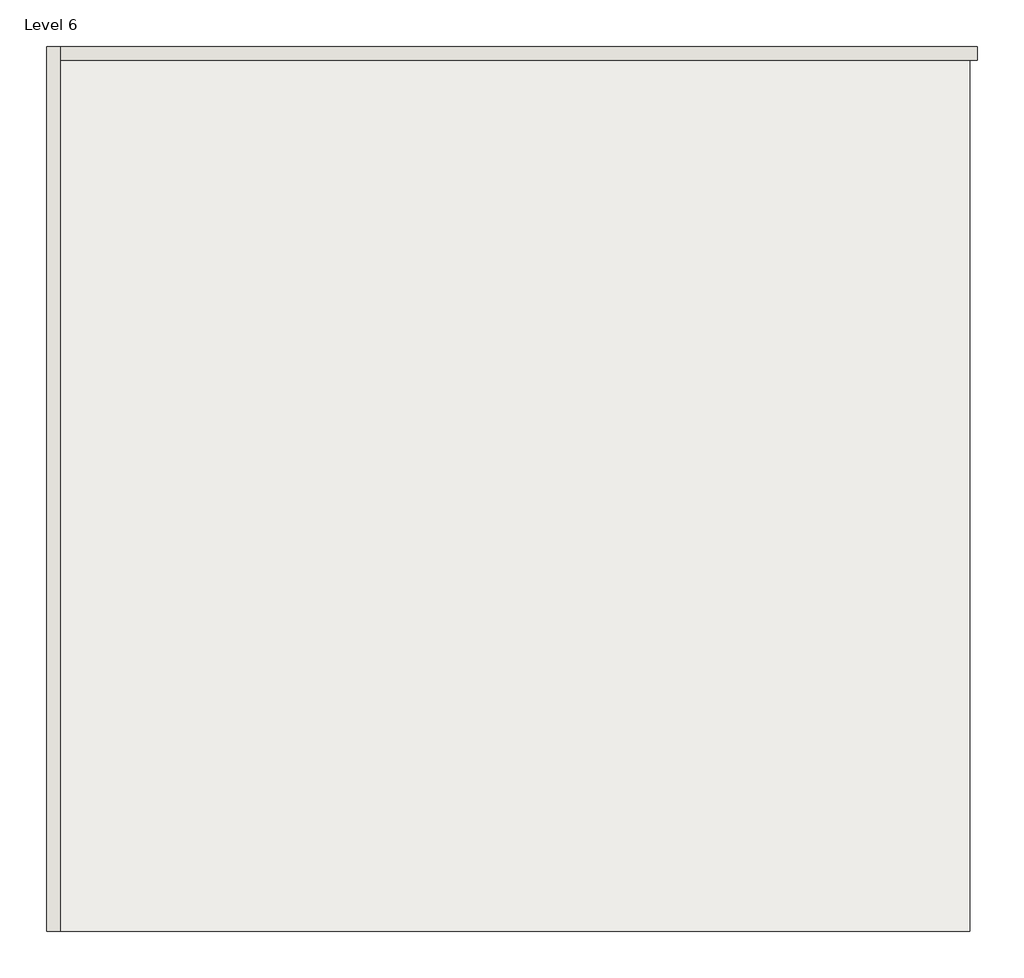
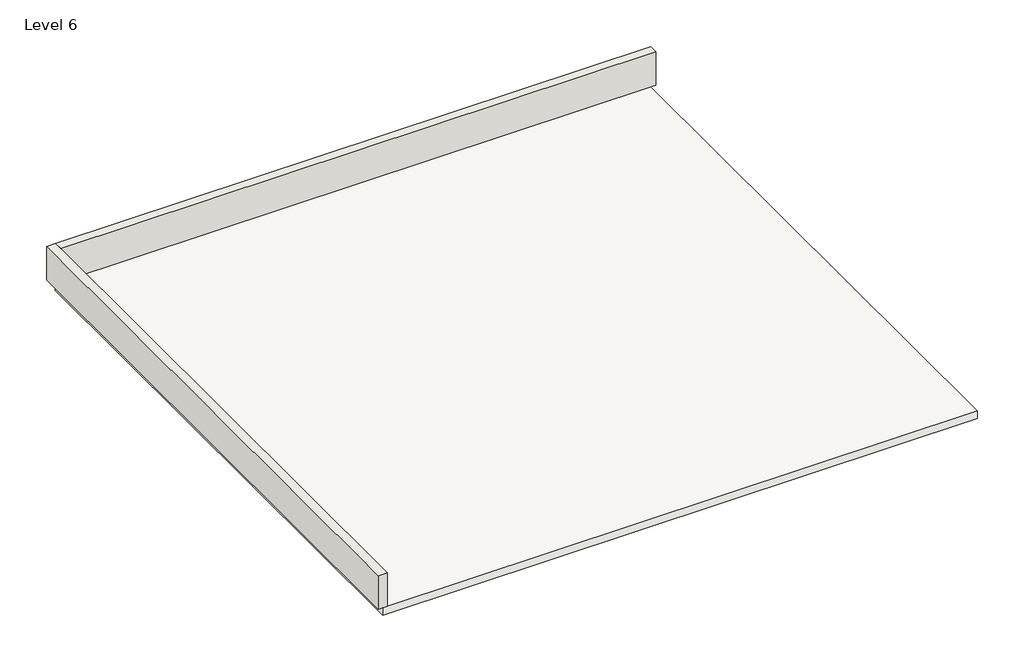
# One storey: 2 walls, 1 slab.
"""IFC4 building model written with IfcOpenShell, lengths in millimetres."""

from ifc_helpers import new_model, si_unit, frame, origin, place, context, project, spatial, polyline, outline, extrude, faceted_brep, element, save

model = new_model("IFC4")

# Units and contexts
model_context = context("Model", 3, world=origin())
ifc_project = project(units=[si_unit("LENGTHUNIT", "METRE", prefix="MILLI")], contexts=[model_context])

# Site, building, storey
site = spatial("IfcSite", under=ifc_project)
building = spatial("IfcBuilding", under=site)
storey = spatial("IfcBuildingStorey", under=building, Name="Level 6", Elevation=16002.0)

# Slab
placement = place(None, origin())
element("IfcSlab", 1, ObjectType="Generic - 12\"", at=placement, inside=storey, context=model_context, shape_type="SweptSolid", body=[
    extrude(outline(polyline([(-4522.1944821, 4915.0176665), (-4522.1944821, -9641.8397804), (-19786.2153052, -9641.8397804), (-19786.2153052, 4915.0176665), (-4522.1944821, 4915.0176665)])), frame((0.0, 0.0, 15798.8), z_axis=(0.0, 0.0, 1.0), x_axis=(1.0, 0.0, 0.0)), (0.0, 0.0, 1.0), 203.2),
])

# Walls
element("IfcWall", 2, ObjectType="Generic - 8\"", at=placement, inside=storey, context=model_context, shape_type="Brep", body=[
    faceted_brep([(-19671.9153052, -9641.8397804, 16002.0), (-19671.9153052, 4874.2602196, 16002.0), (-19671.9153052, 5102.8602196, 16002.0), (-19671.9153052, 5102.8602196, 16916.4), (-19671.9153052, 4874.2602196, 16916.4), (-19671.9153052, -9641.8397804, 16916.4), (-19900.5153052, -9641.8397804, 16002.0), (-19900.5153052, -9641.8397804, 16916.4), (-19900.5153052, 5102.8602196, 16916.4), (-19900.5153052, 5102.8602196, 16002.0)], [[[0, 1, 2, 3, 4, 5]], [[6, 7, 8, 9]], [[2, 1, 0, 6, 9]], [[5, 4, 3, 8, 7]], [[0, 5, 7, 6]], [[3, 2, 9, 8]]]),
])
element("IfcWall", 3, ObjectType="Generic - 8\"", at=placement, inside=storey, context=model_context, shape_type="SweptSolid", body=[
    extrude(outline(polyline([(-4393.8153052, 4874.2602196), (-19671.9153052, 4874.2602196), (-19671.9153052, 5102.8602196), (-4393.8153052, 5102.8602196), (-4393.8153052, 4874.2602196)])), frame((0.0, 0.0, 16002.0), z_axis=(0.0, 0.0, 1.0), x_axis=(1.0, 0.0, 0.0)), (0.0, 0.0, 1.0), 914.4),
])

save(model, "model.ifc")

# Revit data of these elements
# Type "Generic - 12\""
#   Assembly Code = "B1010"
#   Function = 0
#   Layers, outside or top first: 0' - 8" no material (function 1)
# Type "Generic - 8\""
#   Assembly Code = "B2010"
#   Layers, outside or top first: 0' - 9" no material (function 1)
# Element 1 (IfcSlab, "Generic - 12\"")
#   Height Offset From Level = 0' - 0"
#   Phase Created = New Construction
#   Materials on its faces: "Default Floor"
# Elements 2, 3 (IfcWall, "Generic - 8\"")
#   Top Offset = 0' - 0"
#   Base Offset = 0' - 0"
#   Unconnected Height = 3' - 0"
#   wall height = 3' - 0"
#   Phase Created = New Construction
#   Base Constraint = Level 6
#   Materials on its faces: "Default Wall"
# Materials
#   "Default Floor": colour RGB 128 128 128, transparency 0
#   "Default Wall": colour RGB 128 128 128, transparency 0
